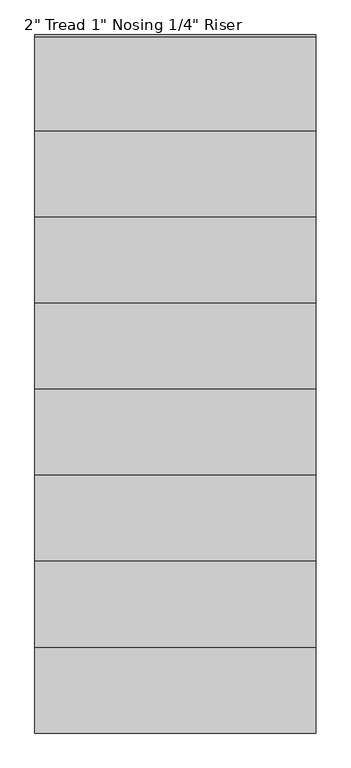
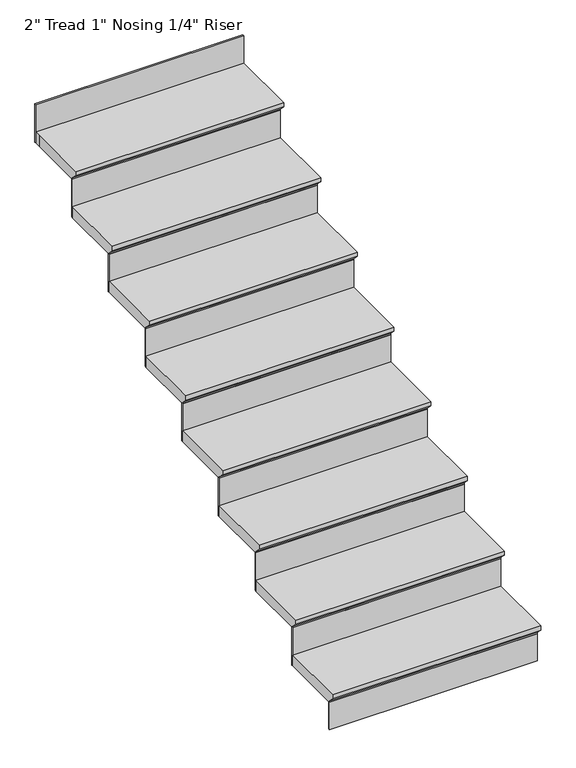
"""IFC4 building model written with IfcOpenShell, lengths in millimetres: stair flight geometry."""

from ifc_helpers import new_model, si_unit, origin, place, context, project, spatial, faceted_brep, source, transform, mapped, element, save


def stair_flight_49f3f953(model_context):
    return source(origin(), model_context, "Body", "Brep", [
        faceted_brep([(-6534.1867944, 11074.6230289, 158.75), (-6534.1867944, 11074.6230289, 177.8), (-7448.5867944, 11074.6230289, 177.8), (-7448.5867944, 11074.6230289, 158.75), (-6534.1867944, 11100.0230289, 133.35), (-7448.5867944, 11100.0230289, 133.35), (-6534.1867944, 11379.4230289, 177.8), (-7448.5867944, 11379.4230289, 177.8), (-7448.5867944, 11100.0230289, 127.0), (-7448.5867944, 11379.4230289, 127.0), (-6534.1867944, 11379.4230289, 127.0), (-6534.1867944, 11100.0230289, 127.0)], [[[0, 1, 2, 3]], [[4, 0, 3, 5]], [[2, 1, 6, 7]], [[8, 9, 10, 11]], [[2, 7, 9, 8, 5, 3]], [[8, 11, 4, 5]], [[6, 1, 0, 4, 11, 10]], [[7, 6, 10, 9]]]),
        faceted_brep([(-6534.1867944, 11100.0230289, 127.0), (-6534.1867944, 11100.0230289, 0.0), (-6534.1867944, 11106.3730289, 0.0), (-6534.1867944, 11106.3730289, 127.0), (-7448.5867944, 11100.0230289, 127.0), (-7448.5867944, 11106.3730289, 127.0), (-7448.5867944, 11106.3730289, 0.0), (-7448.5867944, 11100.0230289, 0.0)], [[[0, 1, 2, 3]], [[4, 5, 6, 7]], [[1, 0, 4, 7]], [[2, 1, 7, 6]], [[3, 2, 6, 5]], [[0, 3, 5, 4]]]),
        faceted_brep([(-6534.1867944, 11379.4230289, 304.8), (-6534.1867944, 11379.4230289, 127.0), (-6534.1867944, 11385.7730289, 127.0), (-6534.1867944, 11385.7730289, 304.8), (-7448.5867944, 11379.4230289, 304.8), (-7448.5867944, 11385.7730289, 304.8), (-7448.5867944, 11385.7730289, 127.0), (-7448.5867944, 11379.4230289, 127.0)], [[[0, 1, 2, 3]], [[4, 5, 6, 7]], [[1, 0, 4, 7]], [[2, 1, 7, 6]], [[3, 2, 6, 5]], [[0, 3, 5, 4]]]),
        faceted_brep([(-7448.5867944, 11354.0230289, 355.6), (-6534.1867944, 11354.0230289, 355.6), (-6534.1867944, 11658.8230289, 355.6), (-7448.5867944, 11658.8230289, 355.6), (-7448.5867944, 11379.4230289, 304.8), (-7448.5867944, 11658.8230289, 304.8), (-6534.1867944, 11658.8230289, 304.8), (-6534.1867944, 11379.4230289, 304.8), (-7448.5867944, 11379.4230289, 311.15), (-7448.5867944, 11354.0230289, 336.55), (-6534.1867944, 11379.4230289, 311.15), (-6534.1867944, 11354.0230289, 336.55)], [[[0, 1, 2, 3]], [[4, 5, 6, 7]], [[0, 3, 5, 4, 8, 9]], [[4, 7, 10, 8]], [[2, 1, 11, 10, 7, 6]], [[3, 2, 6, 5]], [[11, 1, 0, 9]], [[10, 11, 9, 8]]]),
        faceted_brep([(-6534.1867944, 11658.8230289, 482.6), (-6534.1867944, 11658.8230289, 304.8), (-6534.1867944, 11665.1730289, 304.8), (-6534.1867944, 11665.1730289, 482.6), (-7448.5867944, 11658.8230289, 482.6), (-7448.5867944, 11665.1730289, 482.6), (-7448.5867944, 11665.1730289, 304.8), (-7448.5867944, 11658.8230289, 304.8)], [[[0, 1, 2, 3]], [[4, 5, 6, 7]], [[1, 0, 4, 7]], [[2, 1, 7, 6]], [[3, 2, 6, 5]], [[0, 3, 5, 4]]]),
        faceted_brep([(-7448.5867944, 11633.4230289, 533.4), (-6534.1867944, 11633.4230289, 533.4), (-6534.1867944, 11938.2230289, 533.4), (-7448.5867944, 11938.2230289, 533.4), (-7448.5867944, 11658.8230289, 482.6), (-7448.5867944, 11938.2230289, 482.6), (-6534.1867944, 11938.2230289, 482.6), (-6534.1867944, 11658.8230289, 482.6), (-7448.5867944, 11658.8230289, 488.95), (-7448.5867944, 11633.4230289, 514.35), (-6534.1867944, 11658.8230289, 488.95), (-6534.1867944, 11633.4230289, 514.35)], [[[0, 1, 2, 3]], [[4, 5, 6, 7]], [[0, 3, 5, 4, 8, 9]], [[4, 7, 10, 8]], [[2, 1, 11, 10, 7, 6]], [[3, 2, 6, 5]], [[11, 1, 0, 9]], [[10, 11, 9, 8]]]),
        faceted_brep([(-6534.1867944, 11938.2230289, 660.4), (-6534.1867944, 11938.2230289, 482.6), (-6534.1867944, 11944.5730289, 482.6), (-6534.1867944, 11944.5730289, 660.4), (-7448.5867944, 11938.2230289, 660.4), (-7448.5867944, 11944.5730289, 660.4), (-7448.5867944, 11944.5730289, 482.6), (-7448.5867944, 11938.2230289, 482.6)], [[[0, 1, 2, 3]], [[4, 5, 6, 7]], [[1, 0, 4, 7]], [[2, 1, 7, 6]], [[3, 2, 6, 5]], [[0, 3, 5, 4]]]),
        faceted_brep([(-7448.5867944, 11912.8230289, 711.2), (-6534.1867944, 11912.8230289, 711.2), (-6534.1867944, 12217.6230289, 711.2), (-7448.5867944, 12217.6230289, 711.2), (-7448.5867944, 11938.2230289, 660.4), (-7448.5867944, 12217.6230289, 660.4), (-6534.1867944, 12217.6230289, 660.4), (-6534.1867944, 11938.2230289, 660.4), (-7448.5867944, 11938.2230289, 666.75), (-7448.5867944, 11912.8230289, 692.15), (-6534.1867944, 11938.2230289, 666.75), (-6534.1867944, 11912.8230289, 692.15)], [[[0, 1, 2, 3]], [[4, 5, 6, 7]], [[0, 3, 5, 4, 8, 9]], [[4, 7, 10, 8]], [[2, 1, 11, 10, 7, 6]], [[3, 2, 6, 5]], [[11, 1, 0, 9]], [[10, 11, 9, 8]]]),
        faceted_brep([(-6534.1867944, 12217.6230289, 838.2), (-6534.1867944, 12217.6230289, 660.4), (-6534.1867944, 12223.9730289, 660.4), (-6534.1867944, 12223.9730289, 838.2), (-7448.5867944, 12217.6230289, 838.2), (-7448.5867944, 12223.9730289, 838.2), (-7448.5867944, 12223.9730289, 660.4), (-7448.5867944, 12217.6230289, 660.4)], [[[0, 1, 2, 3]], [[4, 5, 6, 7]], [[1, 0, 4, 7]], [[2, 1, 7, 6]], [[3, 2, 6, 5]], [[0, 3, 5, 4]]]),
        faceted_brep([(-7448.5867944, 12192.2230289, 889.0), (-6534.1867944, 12192.2230289, 889.0), (-6534.1867944, 12497.0230289, 889.0), (-7448.5867944, 12497.0230289, 889.0), (-7448.5867944, 12217.6230289, 838.2), (-7448.5867944, 12497.0230289, 838.2), (-6534.1867944, 12497.0230289, 838.2), (-6534.1867944, 12217.6230289, 838.2), (-7448.5867944, 12217.6230289, 844.55), (-7448.5867944, 12192.2230289, 869.95), (-6534.1867944, 12217.6230289, 844.55), (-6534.1867944, 12192.2230289, 869.95)], [[[0, 1, 2, 3]], [[4, 5, 6, 7]], [[0, 3, 5, 4, 8, 9]], [[4, 7, 10, 8]], [[2, 1, 11, 10, 7, 6]], [[3, 2, 6, 5]], [[11, 1, 0, 9]], [[10, 11, 9, 8]]]),
        faceted_brep([(-6534.1867944, 12497.0230289, 1016.0), (-6534.1867944, 12497.0230289, 838.2), (-6534.1867944, 12503.3730289, 838.2), (-6534.1867944, 12503.3730289, 1016.0), (-7448.5867944, 12497.0230289, 1016.0), (-7448.5867944, 12503.3730289, 1016.0), (-7448.5867944, 12503.3730289, 838.2), (-7448.5867944, 12497.0230289, 838.2)], [[[0, 1, 2, 3]], [[4, 5, 6, 7]], [[1, 0, 4, 7]], [[2, 1, 7, 6]], [[3, 2, 6, 5]], [[0, 3, 5, 4]]]),
        faceted_brep([(-7448.5867944, 12471.6230289, 1066.8), (-6534.1867944, 12471.6230289, 1066.8), (-6534.1867944, 12776.4230289, 1066.8), (-7448.5867944, 12776.4230289, 1066.8), (-7448.5867944, 12497.0230289, 1016.0), (-7448.5867944, 12776.4230289, 1016.0), (-6534.1867944, 12776.4230289, 1016.0), (-6534.1867944, 12497.0230289, 1016.0), (-7448.5867944, 12497.0230289, 1022.35), (-7448.5867944, 12471.6230289, 1047.75), (-6534.1867944, 12497.0230289, 1022.35), (-6534.1867944, 12471.6230289, 1047.75)], [[[0, 1, 2, 3]], [[4, 5, 6, 7]], [[0, 3, 5, 4, 8, 9]], [[4, 7, 10, 8]], [[2, 1, 11, 10, 7, 6]], [[3, 2, 6, 5]], [[11, 1, 0, 9]], [[10, 11, 9, 8]]]),
        faceted_brep([(-6534.1867944, 12776.4230289, 1193.8), (-6534.1867944, 12776.4230289, 1016.0), (-6534.1867944, 12782.7730289, 1016.0), (-6534.1867944, 12782.7730289, 1193.8), (-7448.5867944, 12776.4230289, 1193.8), (-7448.5867944, 12782.7730289, 1193.8), (-7448.5867944, 12782.7730289, 1016.0), (-7448.5867944, 12776.4230289, 1016.0)], [[[0, 1, 2, 3]], [[4, 5, 6, 7]], [[1, 0, 4, 7]], [[2, 1, 7, 6]], [[3, 2, 6, 5]], [[0, 3, 5, 4]]]),
        faceted_brep([(-7448.5867944, 12751.0230289, 1244.6), (-6534.1867944, 12751.0230289, 1244.6), (-6534.1867944, 13055.8230289, 1244.6), (-7448.5867944, 13055.8230289, 1244.6), (-7448.5867944, 12776.4230289, 1193.8), (-7448.5867944, 13055.8230289, 1193.8), (-6534.1867944, 13055.8230289, 1193.8), (-6534.1867944, 12776.4230289, 1193.8), (-7448.5867944, 12776.4230289, 1200.15), (-7448.5867944, 12751.0230289, 1225.55), (-6534.1867944, 12776.4230289, 1200.15), (-6534.1867944, 12751.0230289, 1225.55)], [[[0, 1, 2, 3]], [[4, 5, 6, 7]], [[0, 3, 5, 4, 8, 9]], [[4, 7, 10, 8]], [[2, 1, 11, 10, 7, 6]], [[3, 2, 6, 5]], [[11, 1, 0, 9]], [[10, 11, 9, 8]]]),
        faceted_brep([(-6534.1867944, 13335.2230289, 1549.4), (-6534.1867944, 13335.2230289, 1371.6), (-6534.1867944, 13341.5730289, 1371.6), (-6534.1867944, 13341.5730289, 1549.4), (-7448.5867944, 13335.2230289, 1549.4), (-7448.5867944, 13341.5730289, 1549.4), (-7448.5867944, 13341.5730289, 1371.6), (-7448.5867944, 13335.2230289, 1371.6)], [[[0, 1, 2, 3]], [[4, 5, 6, 7]], [[1, 0, 4, 7]], [[2, 1, 7, 6]], [[3, 2, 6, 5]], [[0, 3, 5, 4]]]),
        faceted_brep([(-6534.1867944, 13055.8230289, 1371.6), (-6534.1867944, 13055.8230289, 1193.8), (-6534.1867944, 13062.1730289, 1193.8), (-6534.1867944, 13062.1730289, 1371.6), (-7448.5867944, 13055.8230289, 1371.6), (-7448.5867944, 13062.1730289, 1371.6), (-7448.5867944, 13062.1730289, 1193.8), (-7448.5867944, 13055.8230289, 1193.8)], [[[0, 1, 2, 3]], [[4, 5, 6, 7]], [[1, 0, 4, 7]], [[2, 1, 7, 6]], [[3, 2, 6, 5]], [[0, 3, 5, 4]]]),
        faceted_brep([(-7448.5867944, 13335.2230289, 1422.4), (-7448.5867944, 13309.8230289, 1422.4), (-7448.5867944, 13030.4230289, 1422.4), (-6534.1867944, 13030.4230289, 1422.4), (-6534.1867944, 13335.2230289, 1422.4), (-7448.5867944, 13309.8230289, 1371.6), (-7448.5867944, 13335.2230289, 1371.6), (-6534.1867944, 13335.2230289, 1371.6), (-6534.1867944, 13055.8230289, 1371.6), (-7448.5867944, 13055.8230289, 1371.6), (-7448.5867944, 13055.8230289, 1377.95), (-7448.5867944, 13030.4230289, 1403.35), (-6534.1867944, 13055.8230289, 1377.95), (-6534.1867944, 13030.4230289, 1403.35)], [[[0, 1, 2, 3, 4]], [[5, 6, 7, 8, 9]], [[1, 0, 6, 5]], [[2, 1, 5, 9, 10, 11]], [[9, 8, 12, 10]], [[4, 3, 13, 12, 8, 7]], [[0, 4, 7, 6]], [[13, 3, 2, 11]], [[12, 13, 11, 10]]]),
    ])


if __name__ == "__main__":
    model = new_model("IFC4")
    model_context = context("Model", 3, world=origin())
    ifc_project = project(units=[si_unit("LENGTHUNIT", "METRE", prefix="MILLI")], contexts=[model_context])
    site = spatial("IfcSite", under=ifc_project)
    building = spatial("IfcBuilding", under=site)
    placement = place(None, origin())
    stair_flight_shape = stair_flight_49f3f953(model_context)
    element("IfcStairFlight", 1, ObjectType="2\" Tread 1\" Nosing 1/4\" Riser", at=placement, inside=building, context=model_context, shape_type="MappedRepresentation", body=[
        mapped(stair_flight_shape, transform((0.0, 0.0, 0.0), x_axis=(1.0, 0.0, 0.0), y_axis=(0.0, 1.0, 0.0), z_axis=(0.0, 0.0, 1.0))),
    ])
    save(model, "model.ifc")
